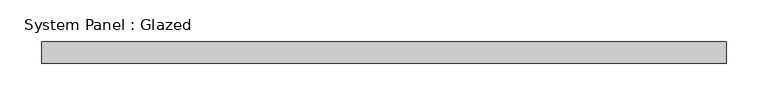
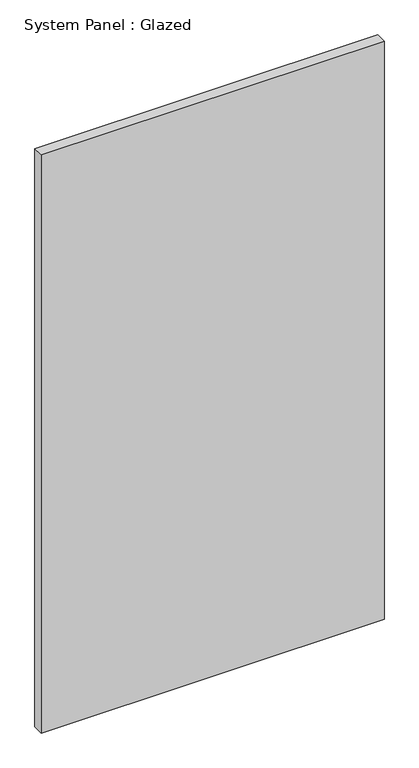
"""IFC4 building model written with IfcOpenShell, lengths in millimetres: plate geometry, System Panel : Glazed."""

from ifc_helpers import new_model, si_unit, origin, origin_with_axes, place, context, project, spatial, polyline, outline, extrude, source, transform, mapped, element, save


def system_panel_glazed_016e6134(model_context):
    return source(origin(), model_context, "Body", "SweptSolid", [
        extrude(outline(polyline([(409.575, 19.05), (-409.575, 19.05), (-409.575, 44.45), (409.575, 44.45), (409.575, 19.05)])), origin_with_axes(), (0.0, 0.0, 1.0), 1460.5),
    ])


if __name__ == "__main__":
    model = new_model("IFC4")
    model_context = context("Model", 3, world=origin())
    ifc_project = project(units=[si_unit("LENGTHUNIT", "METRE", prefix="MILLI")], contexts=[model_context])
    site = spatial("IfcSite", under=ifc_project)
    building = spatial("IfcBuilding", under=site)
    placement = place(None, origin())
    system_panel_glazed_shape = system_panel_glazed_016e6134(model_context)
    element("IfcPlate", 1, ObjectType="System Panel : Glazed", at=placement, inside=building, context=model_context, shape_type="MappedRepresentation", body=[
        mapped(system_panel_glazed_shape, transform((0.0, 0.0, 0.0), x_axis=(1.0, 0.0, 0.0), y_axis=(0.0, 1.0, 0.0), z_axis=(0.0, 0.0, 1.0))),
    ])
    save(model, "model.ifc")

# Revit data of these elements
# Type "System Panel : Glazed"
#   Construction Type Id = "GSP4R"
#   Analytic Construction = "1/8 in Pilkington single glazing"
#   Visual Light Transmittance = 0.9
#   Solar Heat Gain Coefficient = 0.86
#   Heat Transfer Coefficient (U) = 1.18115 BTU/(h·ft²·°F)
#   Define Thermal Properties by = 1
# Element 1 (IfcPlate, "System Panel : Glazed")
#   Materials on its faces: "Glass"
# Materials
#   "Glass": class "Glass", colour RGB 0 128 192, transparency 0.75, Description = "Soda Lime Glass", Cost = 0
